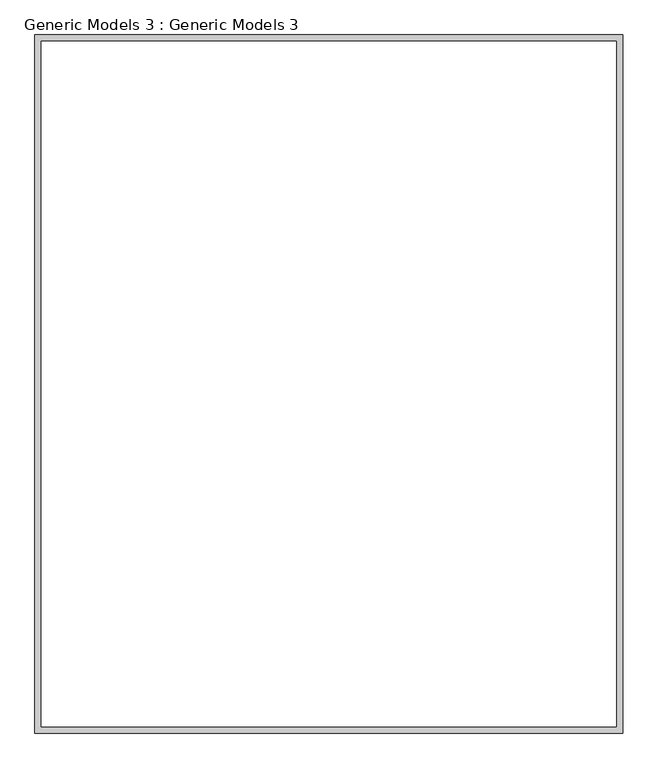
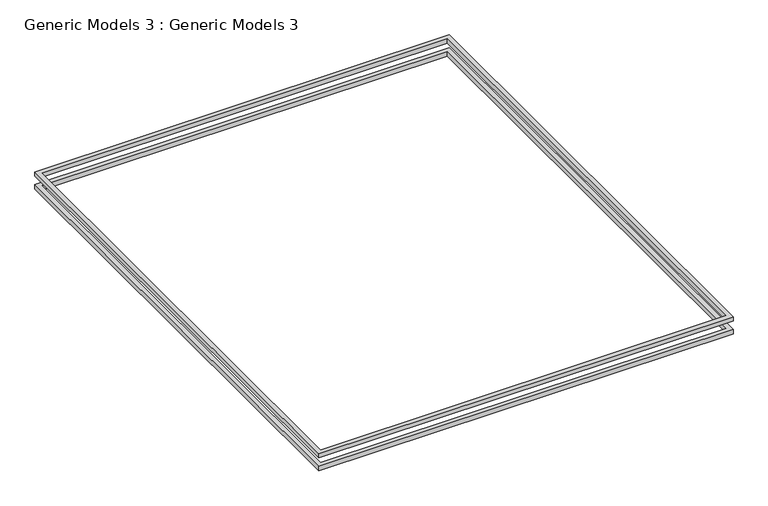
"""IFC4 building model written with IfcOpenShell, lengths in millimetres: proxy geometry, Generic Models 3 : Generic Models 3."""

from ifc_helpers import new_model, si_unit, frame, origin, place, context, project, spatial, polyline, outline, extrude, source, transform, mapped, element, save


def generic_models_3_generic_models_3_31b21ce6(model_context):
    return source(origin(), model_context, "Body", "SweptSolid", [
        extrude(outline(polyline([(-10774.4463366, 1019.7684231), (-10774.4463366, -4530.3968048), (-15448.0463366, -4530.3968048), (-15448.0463366, 1019.7684231), (-10774.4463366, 1019.7684231)]), holes=[polyline([(-15397.2463366, 968.9684231), (-15397.2463366, -4479.5968048), (-10825.2463366, -4479.5968048), (-10825.2463366, 968.9684231), (-15397.2463366, 968.9684231)])]), frame((0.0, 0.0, 10007.6), z_axis=(0.0, 0.0, 1.0), x_axis=(1.0, 0.0, 0.0)), (0.0, 0.0, 1.0), 50.8),
        extrude(outline(polyline([(-10774.4463366, 1019.7684231), (-10774.4463366, -4530.3968048), (-15448.0463366, -4530.3968048), (-15448.0463366, 1019.7684231), (-10774.4463366, 1019.7684231)]), holes=[polyline([(-15397.2463366, 968.9684231), (-15397.2463366, -4479.5968048), (-10825.2463366, -4479.5968048), (-10825.2463366, 968.9684231), (-15397.2463366, 968.9684231)])]), frame((0.0, 0.0, 10160.0), z_axis=(0.0, 0.0, 1.0), x_axis=(1.0, 0.0, 0.0)), (0.0, 0.0, 1.0), 50.8),
    ])


if __name__ == "__main__":
    model = new_model("IFC4")
    model_context = context("Model", 3, world=origin())
    ifc_project = project(units=[si_unit("LENGTHUNIT", "METRE", prefix="MILLI")], contexts=[model_context])
    site = spatial("IfcSite", under=ifc_project)
    building = spatial("IfcBuilding", under=site)
    placement = place(None, origin())
    generic_models_3_generic_models_3_shape = generic_models_3_generic_models_3_31b21ce6(model_context)
    element("IfcBuildingElementProxy", 1, Name="Generic Models 3 : Generic Models 3", ObjectType="Generic Models 3 : Generic Models 3", at=placement, inside=building, context=model_context, shape_type="MappedRepresentation", body=[
        mapped(generic_models_3_generic_models_3_shape, transform((0.0, 0.0, 0.0), x_axis=(1.0, 0.0, 0.0), y_axis=(0.0, 1.0, 0.0), z_axis=(0.0, 0.0, 1.0))),
    ])
    save(model, "model.ifc")

# Revit data of these elements
# Element 1 (IfcBuildingElementProxy, "Generic Models 3 : Generic Models 3")
#   Materials on its faces: "Wood Planks"
# Materials
#   "Wood Planks": class "Wood", colour RGB 129 72 39, transparency 0, Description = "Physical material.", Cost = 0
